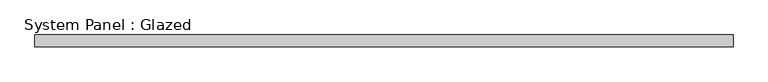
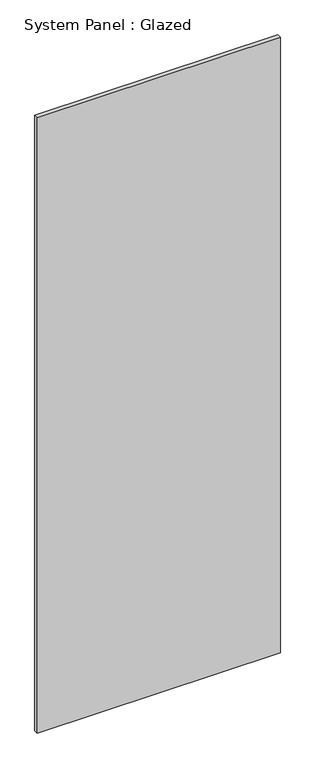
"""IFC4 building model written with IfcOpenShell, lengths in millimetres: plate geometry, System Panel : Glazed."""

from ifc_helpers import new_model, si_unit, origin, origin_with_axes, place, context, project, spatial, polyline, outline, extrude, source, transform, mapped, element, save


def system_panel_glazed_d137d5b4(model_context):
    return source(origin(), model_context, "Body", "SweptSolid", [
        extrude(outline(polyline([(747.9865492, 24.5), (-747.9865492, 24.5), (-747.9865492, 49.5), (747.9865492, 49.5), (747.9865492, 24.5)])), origin_with_axes(), (0.0, 0.0, 1.0), 4000.0),
    ])


if __name__ == "__main__":
    model = new_model("IFC4")
    model_context = context("Model", 3, world=origin())
    ifc_project = project(units=[si_unit("LENGTHUNIT", "METRE", prefix="MILLI")], contexts=[model_context])
    site = spatial("IfcSite", under=ifc_project)
    building = spatial("IfcBuilding", under=site)
    placement = place(None, origin())
    system_panel_glazed_shape = system_panel_glazed_d137d5b4(model_context)
    element("IfcPlate", 1, ObjectType="System Panel : Glazed", at=placement, inside=building, context=model_context, shape_type="MappedRepresentation", body=[
        mapped(system_panel_glazed_shape, transform((0.0, 0.0, 0.0), x_axis=(1.0, 0.0, 0.0), y_axis=(0.0, 1.0, 0.0), z_axis=(0.0, 0.0, 1.0))),
    ])
    save(model, "model.ifc")

# Revit data of these elements
# Type "System Panel : Glazed"
#   Keynote = "H11"
#   Construction Type Id = "GSP4R"
#   Analytic Construction = "1/8 in Pilkington single glazing"
#   Visual Light Transmittance = 0.9
#   Solar Heat Gain Coefficient = 0.86
#   Heat Transfer Coefficient (U) = 6.7069 W/(m²·K)
#   Define Thermal Properties by = 1
# Element 1 (IfcPlate, "System Panel : Glazed")
#   Materials on its faces: "Glass"
# Materials
#   "Glass": class "Glass", colour RGB 0 128 192, transparency 0.9, Description = "Soda Lime Glass", Cost = 0
